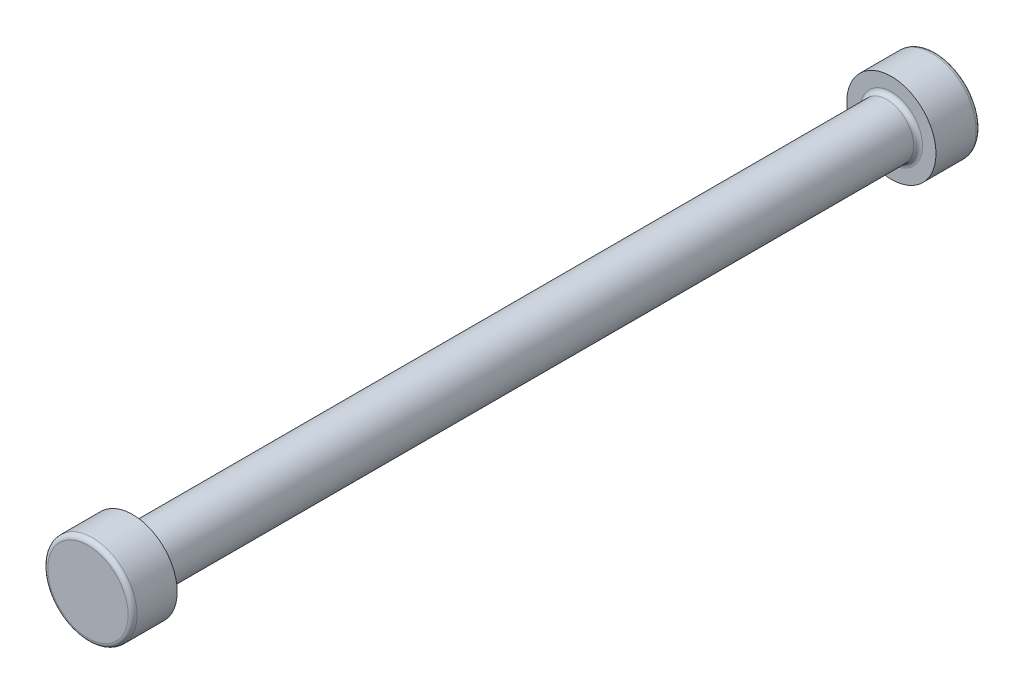
ISO-10303-21;
HEADER;
FILE_DESCRIPTION(('STEP AP214'),'2;1');
FILE_NAME('part.step','',(''),(''),'','','');
FILE_SCHEMA(('AUTOMOTIVE_DESIGN { 1 0 10303 214 1 1 1 1 }'));
ENDSEC;
DATA;
#1=APPLICATION_CONTEXT('core data for automotive mechanical design processes');
#2=APPLICATION_PROTOCOL_DEFINITION('international standard','automotive_design',2000,#1);
#3=PRODUCT_CONTEXT('',#1,'mechanical');
#4=PRODUCT('Part','Part','',(#3));
#5=PRODUCT_RELATED_PRODUCT_CATEGORY('part','',(#4));
#6=PRODUCT_DEFINITION_FORMATION('','',#4);
#7=PRODUCT_DEFINITION_CONTEXT('part definition',#1,'design');
#8=PRODUCT_DEFINITION('design','',#6,#7);
#9=PRODUCT_DEFINITION_SHAPE('','',#8);
#10=(LENGTH_UNIT() NAMED_UNIT(*) SI_UNIT(.MILLI.,.METRE.));
#11=(NAMED_UNIT(*) PLANE_ANGLE_UNIT() SI_UNIT($,.RADIAN.));
#12=(NAMED_UNIT(*) SI_UNIT($,.STERADIAN.) SOLID_ANGLE_UNIT());
#13=UNCERTAINTY_MEASURE_WITH_UNIT(LENGTH_MEASURE(1.E-05),#10,'distance_accuracy_value','');
#14=(GEOMETRIC_REPRESENTATION_CONTEXT(3) GLOBAL_UNCERTAINTY_ASSIGNED_CONTEXT((#13)) GLOBAL_UNIT_ASSIGNED_CONTEXT((#10,
#11,#12)) REPRESENTATION_CONTEXT('',''));
#15=CARTESIAN_POINT('',(0.,0.,0.));
#16=DIRECTION('',(0.,0.,1.));
#17=DIRECTION('',(1.,0.,0.));
#18=AXIS2_PLACEMENT_3D('',#15,#16,#17);
#19=CARTESIAN_POINT('',(0.,0.,47.5));
#20=DIRECTION('',(0.,0.,-1.));
#21=DIRECTION('',(-1.,0.,0.));
#22=AXIS2_PLACEMENT_3D('',#19,#20,#21);
#23=CYLINDRICAL_SURFACE('',#22,3.);
#24=CARTESIAN_POINT('',(0.,0.,-42.));
#25=DIRECTION('',(0.,0.,-1.));
#26=DIRECTION('',(-1.,0.,0.));
#27=AXIS2_PLACEMENT_3D('',#24,#25,#26);
#28=CIRCLE('',#27,3.);
#29=CARTESIAN_POINT('',(-3.,0.,-42.));
#30=VERTEX_POINT('',#29);
#31=EDGE_CURVE('E46',#30,#30,#28,.F.);
#32=ORIENTED_EDGE('',*,*,#31,.T.);
#33=EDGE_LOOP('',(#32));
#34=FACE_BOUND('',#33,.T.);
#35=CARTESIAN_POINT('',(0.,0.,42.));
#36=DIRECTION('',(0.,0.,1.));
#37=DIRECTION('',(1.,0.,0.));
#38=AXIS2_PLACEMENT_3D('',#35,#36,#37);
#39=CIRCLE('',#38,3.);
#40=CARTESIAN_POINT('',(3.,0.,42.));
#41=VERTEX_POINT('',#40);
#42=EDGE_CURVE('E49',#41,#41,#39,.F.);
#43=ORIENTED_EDGE('',*,*,#42,.T.);
#44=EDGE_LOOP('',(#43));
#45=FACE_BOUND('',#44,.T.);
#46=ADVANCED_FACE('F39',(#34,#45),#23,.T.);
#47=CARTESIAN_POINT('',(0.,0.,42.5));
#48=DIRECTION('',(0.,0.,1.));
#49=DIRECTION('',(1.,0.,0.));
#50=AXIS2_PLACEMENT_3D('',#47,#48,#49);
#51=CYLINDRICAL_SURFACE('',#50,5.);
#52=CARTESIAN_POINT('',(0.,0.,47.));
#53=DIRECTION('',(0.,0.,1.));
#54=DIRECTION('',(1.,0.,0.));
#55=AXIS2_PLACEMENT_3D('',#52,#53,#54);
#56=CIRCLE('',#55,5.);
#57=CARTESIAN_POINT('',(5.,0.,47.));
#58=VERTEX_POINT('',#57);
#59=EDGE_CURVE('E56',#58,#58,#56,.F.);
#60=ORIENTED_EDGE('',*,*,#59,.T.);
#61=EDGE_LOOP('',(#60));
#62=FACE_BOUND('',#61,.T.);
#63=CARTESIAN_POINT('',(0.,0.,42.5));
#64=DIRECTION('',(0.,0.,1.));
#65=DIRECTION('',(1.,0.,0.));
#66=AXIS2_PLACEMENT_3D('',#63,#64,#65);
#67=CIRCLE('',#66,5.);
#68=CARTESIAN_POINT('',(5.,0.,42.5));
#69=VERTEX_POINT('',#68);
#70=EDGE_CURVE('E72',#69,#69,#67,.T.);
#71=ORIENTED_EDGE('',*,*,#70,.T.);
#72=EDGE_LOOP('',(#71));
#73=FACE_BOUND('',#72,.T.);
#74=ADVANCED_FACE('F100',(#62,#73),#51,.T.);
#75=CARTESIAN_POINT('',(0.,0.,42.5));
#76=DIRECTION('',(0.,0.,1.));
#77=DIRECTION('',(1.,0.,0.));
#78=AXIS2_PLACEMENT_3D('',#75,#76,#77);
#79=PLANE('',#78);
#80=CARTESIAN_POINT('',(0.,0.,42.5));
#81=DIRECTION('',(0.,0.,1.));
#82=DIRECTION('',(1.,0.,0.));
#83=AXIS2_PLACEMENT_3D('',#80,#81,#82);
#84=CIRCLE('',#83,3.5);
#85=CARTESIAN_POINT('',(3.5,0.,42.5));
#86=VERTEX_POINT('',#85);
#87=EDGE_CURVE('E10',#86,#86,#84,.T.);
#88=ORIENTED_EDGE('',*,*,#87,.T.);
#89=EDGE_LOOP('',(#88));
#90=FACE_BOUND('',#89,.T.);
#91=ORIENTED_EDGE('',*,*,#70,.F.);
#92=EDGE_LOOP('',(#91));
#93=FACE_BOUND('',#92,.T.);
#94=ADVANCED_FACE('F95',(#90,#93),#79,.F.);
#95=CARTESIAN_POINT('',(0.,0.,47.5));
#96=DIRECTION('',(0.,0.,1.));
#97=DIRECTION('',(1.,0.,0.));
#98=AXIS2_PLACEMENT_3D('',#95,#96,#97);
#99=PLANE('',#98);
#100=CARTESIAN_POINT('',(0.,0.,47.5));
#101=DIRECTION('',(0.,0.,1.));
#102=DIRECTION('',(1.,0.,0.));
#103=AXIS2_PLACEMENT_3D('',#100,#101,#102);
#104=CIRCLE('',#103,4.5);
#105=CARTESIAN_POINT('',(4.5,0.,47.5));
#106=VERTEX_POINT('',#105);
#107=EDGE_CURVE('E62',#106,#106,#104,.T.);
#108=ORIENTED_EDGE('',*,*,#107,.T.);
#109=EDGE_LOOP('',(#108));
#110=FACE_BOUND('',#109,.T.);
#111=ADVANCED_FACE('F84',(#110),#99,.T.);
#112=CARTESIAN_POINT('',(0.,0.,-42.5));
#113=DIRECTION('',(0.,0.,-1.));
#114=DIRECTION('',(-1.,0.,0.));
#115=AXIS2_PLACEMENT_3D('',#112,#113,#114);
#116=CYLINDRICAL_SURFACE('',#115,5.);
#117=CARTESIAN_POINT('',(0.,0.,-47.));
#118=DIRECTION('',(0.,0.,1.));
#119=DIRECTION('',(1.,0.,0.));
#120=AXIS2_PLACEMENT_3D('',#117,#118,#119);
#121=CIRCLE('',#120,5.);
#122=CARTESIAN_POINT('',(5.,0.,-47.));
#123=VERTEX_POINT('',#122);
#124=EDGE_CURVE('E70',#123,#123,#121,.T.);
#125=ORIENTED_EDGE('',*,*,#124,.T.);
#126=EDGE_LOOP('',(#125));
#127=FACE_BOUND('',#126,.T.);
#128=CARTESIAN_POINT('',(0.,0.,-42.5));
#129=DIRECTION('',(0.,0.,1.));
#130=DIRECTION('',(1.,0.,0.));
#131=AXIS2_PLACEMENT_3D('',#128,#129,#130);
#132=CIRCLE('',#131,5.);
#133=CARTESIAN_POINT('',(5.,0.,-42.5));
#134=VERTEX_POINT('',#133);
#135=EDGE_CURVE('E74',#134,#134,#132,.T.);
#136=ORIENTED_EDGE('',*,*,#135,.F.);
#137=EDGE_LOOP('',(#136));
#138=FACE_BOUND('',#137,.T.);
#139=ADVANCED_FACE('F80',(#127,#138),#116,.T.);
#140=CARTESIAN_POINT('',(0.,0.,-42.5));
#141=DIRECTION('',(0.,0.,-1.));
#142=DIRECTION('',(1.,0.,0.));
#143=AXIS2_PLACEMENT_3D('',#140,#141,#142);
#144=PLANE('',#143);
#145=CARTESIAN_POINT('',(0.,0.,-42.5));
#146=DIRECTION('',(0.,0.,-1.));
#147=DIRECTION('',(-1.,0.,0.));
#148=AXIS2_PLACEMENT_3D('',#145,#146,#147);
#149=CIRCLE('',#148,3.5);
#150=CARTESIAN_POINT('',(-3.5,0.,-42.5));
#151=VERTEX_POINT('',#150);
#152=EDGE_CURVE('E53',#151,#151,#149,.T.);
#153=ORIENTED_EDGE('',*,*,#152,.T.);
#154=EDGE_LOOP('',(#153));
#155=FACE_BOUND('',#154,.T.);
#156=ORIENTED_EDGE('',*,*,#135,.T.);
#157=EDGE_LOOP('',(#156));
#158=FACE_BOUND('',#157,.T.);
#159=ADVANCED_FACE('F79',(#155,#158),#144,.F.);
#160=CARTESIAN_POINT('',(0.,0.,-47.5));
#161=DIRECTION('',(0.,0.,1.));
#162=DIRECTION('',(1.,0.,0.));
#163=AXIS2_PLACEMENT_3D('',#160,#161,#162);
#164=PLANE('',#163);
#165=CARTESIAN_POINT('',(0.,0.,-47.5));
#166=DIRECTION('',(0.,0.,1.));
#167=DIRECTION('',(1.,0.,0.));
#168=AXIS2_PLACEMENT_3D('',#165,#166,#167);
#169=CIRCLE('',#168,4.5);
#170=CARTESIAN_POINT('',(4.5,0.,-47.5));
#171=VERTEX_POINT('',#170);
#172=EDGE_CURVE('E65',#171,#171,#169,.F.);
#173=ORIENTED_EDGE('',*,*,#172,.T.);
#174=EDGE_LOOP('',(#173));
#175=FACE_BOUND('',#174,.T.);
#176=ADVANCED_FACE('F90',(#175),#164,.F.);
#177=CARTESIAN_POINT('',(0.,0.,-47.));
#178=DIRECTION('',(0.,0.,1.));
#179=DIRECTION('',(1.,0.,0.));
#180=AXIS2_PLACEMENT_3D('',#177,#178,#179);
#181=TOROIDAL_SURFACE('',#180,4.5,0.5);
#182=ORIENTED_EDGE('',*,*,#172,.F.);
#183=EDGE_LOOP('',(#182));
#184=FACE_BOUND('',#183,.T.);
#185=ORIENTED_EDGE('',*,*,#124,.F.);
#186=EDGE_LOOP('',(#185));
#187=FACE_BOUND('',#186,.T.);
#188=ADVANCED_FACE('F110',(#184,#187),#181,.T.);
#189=CARTESIAN_POINT('',(0.,0.,47.));
#190=DIRECTION('',(0.,0.,1.));
#191=DIRECTION('',(1.,0.,0.));
#192=AXIS2_PLACEMENT_3D('',#189,#190,#191);
#193=TOROIDAL_SURFACE('',#192,4.5,0.5);
#194=ORIENTED_EDGE('',*,*,#59,.F.);
#195=EDGE_LOOP('',(#194));
#196=FACE_BOUND('',#195,.T.);
#197=ORIENTED_EDGE('',*,*,#107,.F.);
#198=EDGE_LOOP('',(#197));
#199=FACE_BOUND('',#198,.T.);
#200=ADVANCED_FACE('F109',(#196,#199),#193,.T.);
#201=CARTESIAN_POINT('',(0.,0.,-42.));
#202=DIRECTION('',(0.,0.,-1.));
#203=DIRECTION('',(-1.,0.,0.));
#204=AXIS2_PLACEMENT_3D('',#201,#202,#203);
#205=TOROIDAL_SURFACE('',#204,3.5,0.5);
#206=ORIENTED_EDGE('',*,*,#31,.F.);
#207=EDGE_LOOP('',(#206));
#208=FACE_BOUND('',#207,.T.);
#209=ORIENTED_EDGE('',*,*,#152,.F.);
#210=EDGE_LOOP('',(#209));
#211=FACE_BOUND('',#210,.T.);
#212=ADVANCED_FACE('F114',(#208,#211),#205,.F.);
#213=CARTESIAN_POINT('',(0.,0.,42.));
#214=DIRECTION('',(0.,0.,1.));
#215=DIRECTION('',(1.,0.,0.));
#216=AXIS2_PLACEMENT_3D('',#213,#214,#215);
#217=TOROIDAL_SURFACE('',#216,3.5,0.5);
#218=ORIENTED_EDGE('',*,*,#42,.F.);
#219=EDGE_LOOP('',(#218));
#220=FACE_BOUND('',#219,.T.);
#221=ORIENTED_EDGE('',*,*,#87,.F.);
#222=EDGE_LOOP('',(#221));
#223=FACE_BOUND('',#222,.T.);
#224=ADVANCED_FACE('F41',(#220,#223),#217,.F.);
#225=CLOSED_SHELL('',(#46,#74,#94,#111,#139,#159,#176,#188,#200,#212,#224));
#226=MANIFOLD_SOLID_BREP('B2',#225);
#227=ADVANCED_BREP_SHAPE_REPRESENTATION('',(#18,#226),#14);
#228=SHAPE_DEFINITION_REPRESENTATION(#9,#227);
ENDSEC;
END-ISO-10303-21;
